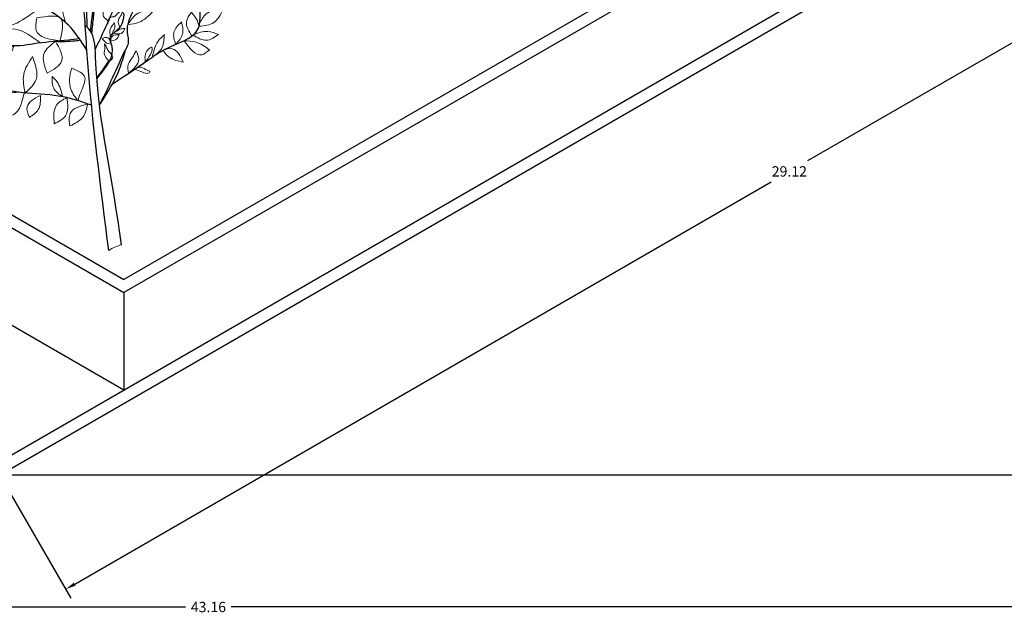
# Model space of a CAD drawing. Units: metres. Extents: x 12735 to 25554, y 20954 to 41989.
# Tile 10 of 15: x 12756 to 12773, y 20954 to 20964. Entities that reach past the tile are written whole.
import ezdxf

# ---------------------------------------------------------------- set-up
doc = ezdxf.new("R2010")
doc.units = ezdxf.units.M
doc.layers.get('Defpoints').update_dxf_attribs({"lineweight": 13})
for name, color, linetype, lineweight in [('A-ANNO-DIMS', 2, 'Continuous', 18), ('C-SITE', 8, 'Continuous', 25), ('TREES', 72, 'Continuous', 18)]:
    doc.layers.add(name, color=color, linetype=linetype, lineweight=lineweight)
doc.layers.add('STEM', color=32, linetype='Continuous')
doc.styles.get("Standard").update_dxf_attribs({"font": 'arial.ttf'})
doc.dimstyles.get("Standard").update_dxf_attribs({"dimtxt": 0.18, "dimasz": 0.18, "dimexe": 0.18, "dimexo": 0.0625, "dimgap": 0.09, "dimtad": 0, "dimtih": 1, "dimtoh": 1, "dimdec": 4, "dimzin": 0, "dimdsep": 46, "dimtxsty": 'Standard', "dimcen": 0.09, "dimadec": 0, "dimazin": 0, "dimtfac": 1, "dimtdec": 4, "dimtofl": 0, "dimtmove": 0, "dimatfit": 3, "dimfxl": 1, "dimtolj": 1, "dimtzin": 0, "dimarcsym": 0})

# ---------------------------------------------------------------- blocks, each defined once
blk = doc.blocks.new('TREES')
blk.add_line((12743.7, 20972.648), (12743.7, 20972.648))
at = {"layer": 'STEM'}
for points, knots in [([(12743.791, 20972.546), (12743.793, 20972.564), (12743.795, 20972.582), (12743.797, 20972.6), (12743.801, 20972.637), (12743.806, 20972.674), (12743.81, 20972.711), (12743.845, 20973.018), (12743.938, 20973.826), (12743.743, 20974.806), (12743.607, 20975.634), (12743.413, 20975.893), (12743.333, 20975.999)], [-0.164913, -0.164913, -0.164913, -0.164913, -0.110972, -0.110972, -0.110972, 0, 0, 0, 0.920963, 2.426088, 2.990404, 3.384799, 3.384799, 3.384799, 3.384799]), ([(12743.7, 20972.648), (12743.691, 20972.807), (12743.671, 20973.194), (12743.257, 20973.699), (12743.111, 20974.379), (12743.038, 20974.998), (12742.993, 20975.377), (12742.974, 20975.54)], [0, 0, 0, 0, 0.469346, 1.137622, 1.869488, 2.521439, 3.013071, 3.013071, 3.013071, 3.013071]), ([(12743.874, 20972.227), (12743.898, 20972.277), (12743.921, 20972.328), (12743.945, 20972.378), (12744.022, 20972.541), (12744.105, 20972.717), (12744.205, 20972.963), (12744.312, 20973.088), (12744.183, 20973.501), (12744.667, 20973.973), (12744.707, 20974.64), (12744.896, 20975.012), (12744.823, 20975.434), (12744.85, 20975.23), (12744.867, 20975.1)], [-0.166951, -0.166951, -0.166951, -0.166951, 0, 0, 0, 0.539768, 0.582066, 0.798222, 0.98781, 1.7696, 2.524754, 2.899414, 3.105113, 3.460848, 3.460848, 3.460848, 3.460848]), ([(12743.728, 20972.218), (12743.63, 20972.372), (12743.383, 20972.76), (12742.753, 20973.07), (12742.291, 20973.419), (12741.984, 20973.759), (12741.959, 20974.098), (12741.675, 20974.346), (12741.563, 20974.543), (12741.494, 20974.663)], [0, 0, 0, 0, 0.542161, 1.359078, 2.03444, 2.290187, 2.703676, 2.968549, 3.382864, 3.382864, 3.382864, 3.382864]), ([(12743.967, 20971.294), (12743.987, 20971.335), (12744.006, 20971.376), (12744.026, 20971.417), (12744.057, 20971.483), (12744.088, 20971.549), (12744.119, 20971.615), (12744.196, 20971.778), (12744.279, 20971.954), (12744.378, 20972.2), (12744.486, 20972.325), (12744.357, 20972.738), (12744.836, 20973.215), (12744.895, 20973.862), (12745.051, 20974.269), (12745.045, 20974.62), (12744.834, 20974.67), (12744.7, 20974.701)], [-0.355099, -0.355099, -0.355099, -0.355099, -0.218492, -0.218492, -0.218492, 0, 0, 0, 0.539768, 0.582066, 0.798222, 0.98781, 1.7696, 2.524754, 2.899414, 3.105113, 3.460848, 3.460848, 3.460848, 3.460848]), ([(12744.175, 20971.633), (12744.383, 20971.767), (12744.692, 20971.967), (12745.149, 20972.305), (12745.828, 20972.463), (12745.606, 20973.185), (12745.967, 20973.583), (12745.99, 20973.882), (12746.002, 20974.029)], [0, 0, 0, 0, 0.736164, 1.094646, 1.754618, 2.392389, 2.840214, 3.27091, 3.27091, 3.27091, 3.27091]), ([(12743.381, 20973.588), (12743.52, 20973.4), (12743.728, 20973.118), (12743.725, 20972.776), (12743.724, 20972.661), (12743.724, 20972.661), (12743.724, 20972.661), (12743.724, 20972.661), (12743.724, 20972.65), (12743.724, 20972.639), (12743.724, 20972.627)], [0, 0, 0, 0, 0.673099, 1.009429, 1.009429, 1.009429, 1.009429, 1.009429, 1.009429, 1.043412, 1.043412, 1.043412, 1.043412]), ([(12743.814, 20972.505), (12743.817, 20972.531), (12743.819, 20972.556), (12743.822, 20972.581), (12743.827, 20972.63), (12743.832, 20972.679), (12743.838, 20972.727), (12743.847, 20972.813), (12743.865, 20972.982), (12743.864, 20973.152), (12743.864, 20973.236)], [-0.2227932, -0.2227932, -0.2227932, -0.2227932, -0.1464713, -0.1464713, -0.1464713, 0, 0, 0, 0.2578951, 0.5103882, 0.5103882, 0.5103882, 0.5103882]), ([(12743.902, 20971.717), (12743.93, 20971.754), (12743.959, 20971.791), (12743.988, 20971.829), (12743.988, 20971.829), (12743.988, 20971.829), (12743.988, 20971.829), (12744.096, 20971.973), (12744.236, 20972.16), (12744.082, 20972.476), (12744.347, 20972.598), (12744.368, 20972.766), (12744.376, 20972.837)], [-0.129757, -0.129757, -0.129757, -0.129757, 0, 0, 0, 0, 0, 0, 0.485118, 0.62751, 0.913144, 1.120766, 1.120766, 1.120766, 1.120766]), ([(12744.111, 20968.725), (12743.967, 20969.837), (12743.799, 20971.142), (12743.712, 20972.453), (12743.7, 20972.648)], [0, 0, 0, 0, 3.359203, 3.944548, 3.944548, 3.944548, 3.944548]), ([(12744.332, 20968.825), (12744.189, 20969.936), (12743.871, 20971.161), (12743.872, 20972.51), (12743.7, 20972.648)], [0, 0, 0, 0, 3.359203, 3.972384, 3.972384, 3.972384, 3.972384]), ([(12743.597, 20972.418), (12743.533, 20972.41), (12743.292, 20972.379), (12742.889, 20972.351), (12742.364, 20972.241), (12741.803, 20972.489), (12741.157, 20972.302), (12740.698, 20972.258), (12740.474, 20972.237)], [0, 0, 0, 0, 0.193148, 0.727923, 1.218416, 1.762371, 2.471743, 3.152626, 3.152626, 3.152626, 3.152626]), ([(12743.181, 20972.372), (12743.296, 20972.37), (12743.441, 20972.368), (12743.583, 20972.39), (12743.613, 20972.395)], [0, 0, 0, 0, 0.3435042, 0.4329772, 0.4329772, 0.4329772, 0.4329772]), ([(12743.948, 20971.264), (12743.975, 20971.305), (12744.002, 20971.345), (12744.029, 20971.386), (12744.029, 20971.386), (12744.029, 20971.386), (12744.029, 20971.386), (12744.129, 20971.55), (12744.289, 20971.812), (12744.368, 20972.107), (12744.398, 20972.218)], [-0.148605, -0.148605, -0.148605, -0.148605, 0, 0, 0, 0, 0, 0, 0.572176, 0.914425, 0.914425, 0.914425, 0.914425]), ([(12743.901, 20971.729), (12743.929, 20971.768), (12743.958, 20971.808), (12743.986, 20971.847), (12743.986, 20971.847), (12743.986, 20971.847), (12743.986, 20971.847), (12744.02, 20971.892), (12744.062, 20971.951), (12744.099, 20972.014), (12744.107, 20972.028)], [-0.1467707, -0.1467707, -0.1467707, -0.1467707, 0, 0, 0, 0, 0, 0, 0.1684242, 0.2179474, 0.2179474, 0.2179474, 0.2179474]), ([(12743.81, 20971.258), (12743.646, 20971.316), (12743.283, 20971.443), (12742.486, 20971.453), (12741.888, 20971.61), (12741.494, 20971.714)], [0, 0, 0, 0, 0.519056, 1.146346, 2.366016, 2.366016, 2.366016, 2.366016])]:
    blk.add_open_spline(points, degree=3, knots=knots, dxfattribs=at)
blk.add_open_spline([(12744.644, 20971.941), (12744.672, 20971.961), (12744.701, 20971.98), (12744.73, 20972)], degree=3, dxfattribs=at)
at = {"layer": 'TREES'}
for points, knots in [([(12743.584, 20975.586), (12743.37, 20975.718), (12743.075, 20975.9), (12743.022, 20976.725), (12743.333, 20976.097), (12743.574, 20975.612)], [0, 0, 0, 0, 0.724771, 1.002271, 1.932196, 1.932196, 1.932196, 1.932196]), ([(12743.021, 20975.14), (12742.985, 20975.224), (12742.928, 20975.356), (12742.766, 20975.539), (12742.854, 20975.638), (12742.901, 20975.69)], [0, 0, 0, 0, 0.2845416, 0.4465287, 0.6279758, 0.6279758, 0.6279758, 0.6279758]), ([(12743.021, 20975.14), (12743.019, 20975.277), (12743.016, 20975.483), (12742.921, 20975.662), (12742.889, 20975.721)], [0, 0, 0, 0, 0.4023849, 0.6031293, 0.6031293, 0.6031293, 0.6031293]), ([(12743.718, 20974.979), (12743.671, 20975.164), (12743.598, 20975.454), (12743.323, 20975.534), (12743.223, 20975.563)], [0, 0, 0, 0, 0.519429, 0.8155501, 0.8155501, 0.8155501, 0.8155501]), ([(12743.223, 20975.563), (12743.266, 20975.448), (12743.36, 20975.195), (12743.592, 20975.055), (12743.718, 20974.979)], [0, 0, 0, 0, 0.3595778, 0.7860105, 0.7860105, 0.7860105, 0.7860105]), ([(12743.737, 20974.871), (12743.729, 20975.055), (12743.718, 20975.333), (12743.914, 20975.516), (12743.981, 20975.578)], [0, 0, 0, 0, 0.5134638, 0.7779111, 0.7779111, 0.7779111, 0.7779111]), ([(12743.737, 20974.871), (12743.801, 20974.971), (12743.939, 20975.186), (12743.966, 20975.441), (12743.981, 20975.578)], [0, 0, 0, 0, 0.351068, 0.7565079, 0.7565079, 0.7565079, 0.7565079]), ([(12744.796, 20974.806), (12744.757, 20974.909), (12744.688, 20975.088), (12744.514, 20975.28), (12744.523, 20975.414), (12744.526, 20975.464)], [0, 0, 0, 0, 0.3323117, 0.5782809, 0.7232611, 0.7232611, 0.7232611, 0.7232611]), ([(12744.805, 20974.813), (12744.804, 20974.918), (12744.803, 20975.076), (12744.822, 20975.37), (12744.643, 20975.427), (12744.526, 20975.464)], [0, 0, 0, 0, 0.3224266, 0.4885617, 0.8037384, 0.8037384, 0.8037384, 0.8037384]), ([(12741.648, 20974.411), (12741.519, 20974.547), (12741.281, 20974.798), (12741.642, 20974.995), (12741.673, 20975.511), (12741.684, 20975.149), (12741.787, 20975.033), (12741.768, 20974.824), (12741.781, 20974.575), (12741.641, 20974.411), (12741.569, 20974.326)], [0, 0, 0, 0, 0.446457, 0.821839, 1.096823, 1.294203, 1.491123, 1.594729, 1.894892, 2.216107, 2.216107, 2.216107, 2.216107]), ([(12743.07, 20974.733), (12742.98, 20974.863), (12742.848, 20975.053), (12742.433, 20975.446), (12742.649, 20974.915), (12742.651, 20974.573), (12742.961, 20974.576), (12743.034, 20974.678), (12743.071, 20974.73)], [0, 0, 0, 0, 0.54832, 0.799685, 1.166614, 1.565159, 1.742127, 1.925713, 1.925713, 1.925713, 1.925713]), ([(12743.031, 20975.058), (12743.048, 20975.139), (12743.077, 20975.281), (12743.184, 20975.377), (12743.231, 20975.418)], [0, 0, 0, 0, 0.2398723, 0.4207027, 0.4207027, 0.4207027, 0.4207027]), ([(12743.037, 20975.007), (12743.075, 20975.058), (12743.166, 20975.181), (12743.207, 20975.33), (12743.231, 20975.418)], [0, 0, 0, 0, 0.1895117, 0.457602, 0.457602, 0.457602, 0.457602]), ([(12744.796, 20974.806), (12744.882, 20974.878), (12745.017, 20974.992), (12745.211, 20975.15), (12745.228, 20975.277), (12745.236, 20975.337)], [0, 0, 0, 0, 0.3416822, 0.5370609, 0.7122352, 0.7122352, 0.7122352, 0.7122352]), ([(12744.839, 20974.951), (12744.859, 20975.055), (12744.903, 20975.272), (12745.122, 20975.315), (12745.236, 20975.337)], [0, 0, 0, 0, 0.2913456, 0.6064398, 0.6064398, 0.6064398, 0.6064398]), ([(12743.814, 20974.4), (12743.798, 20974.494), (12743.764, 20974.693), (12744.115, 20975.006), (12744.156, 20974.79), (12744.01, 20974.677), (12743.989, 20974.434), (12743.864, 20974.438), (12743.809, 20974.439)], [0, 0, 0, 0, 0.311146, 0.650746, 0.669061, 0.940573, 1.125337, 1.270427, 1.270427, 1.270427, 1.270427]), ([(12743.191, 20974.047), (12743.14, 20974.139), (12743.026, 20974.346), (12743.367, 20974.877), (12743.354, 20974.597), (12743.309, 20974.413), (12743.358, 20974.125), (12743.218, 20974.059), (12743.191, 20974.047)], [0, 0, 0, 0, 0.337622, 0.758697, 0.837919, 1.040495, 1.406258, 1.489574, 1.489574, 1.489574, 1.489574]), ([(12744.509, 20973.941), (12744.486, 20974.093), (12744.451, 20974.322), (12744.425, 20974.623), (12744.504, 20974.731), (12744.534, 20974.773)], [0, 0, 0, 0, 0.4681587, 0.7056034, 0.8580265, 0.8580265, 0.8580265, 0.8580265]), ([(12744.534, 20974.773), (12744.556, 20974.698), (12744.634, 20974.425), (12744.562, 20974.144), (12744.509, 20973.941)], [0, 0, 0, 0, 0.2327329, 0.8431329, 0.8431329, 0.8431329, 0.8431329]), ([(12742.028, 20973.754), (12742.003, 20973.912), (12741.953, 20974.218), (12742.174, 20974.414), (12742.283, 20974.81), (12742.258, 20974.48), (12742.304, 20974.323), (12742.246, 20974.069), (12742.227, 20973.932), (12742.006, 20973.671), (12742.066, 20973.72), (12742.075, 20973.727)], [0, 0, 0, 0, 0.436736, 0.842969, 1.012738, 1.21393, 1.403734, 1.613178, 1.897283, 2.067562, 2.097274, 2.097274, 2.097274, 2.097274]), ([(12743.835, 20974.249), (12743.789, 20974.346), (12743.724, 20974.484), (12743.556, 20974.594), (12743.468, 20974.601), (12743.424, 20974.604)], [0, 0, 0, 0, 0.3158223, 0.4463774, 0.5774617, 0.5774617, 0.5774617, 0.5774617]), ([(12743.424, 20974.604), (12743.442, 20974.527), (12743.487, 20974.324), (12743.715, 20974.191), (12743.841, 20974.206), (12743.841, 20974.206)], [0, 0, 0, 0, 0.2361186, 0.6165307, 0.6167763, 0.6167763, 0.6167763, 0.6167763]), ([(12744.554, 20973.975), (12744.669, 20974.016), (12744.893, 20974.094), (12745.019, 20974.421), (12745.06, 20974.624), (12745.08, 20974.72)], [0, 0, 0, 0, 0.348929, 0.678298, 0.9763146, 0.9763146, 0.9763146, 0.9763146]), ([(12744.618, 20974.118), (12744.717, 20974.268), (12744.844, 20974.462), (12745.022, 20974.606), (12745.062, 20974.638)], [0, 0, 0, 0, 0.5333846, 0.686651, 0.686651, 0.686651, 0.686651]), ([(12744.97, 20974.043), (12744.931, 20974.146), (12744.862, 20974.325), (12744.688, 20974.517), (12744.697, 20974.651), (12744.7, 20974.701)], [0, 0, 0, 0, 0.3323117, 0.5782809, 0.7232611, 0.7232611, 0.7232611, 0.7232611]), ([(12745.957, 20973.706), (12745.908, 20973.835), (12745.798, 20974.123), (12745.864, 20974.427), (12745.9, 20974.594)], [0, 0, 0, 0, 0.4051126, 0.906838, 0.906838, 0.906838, 0.906838]), ([(12745.9, 20974.594), (12745.955, 20974.471), (12746.037, 20974.287), (12746.01, 20974.092), (12746.002, 20974.029)], [0, 0, 0, 0, 0.3943838, 0.5836156, 0.5836156, 0.5836156, 0.5836156]), ([(12744.97, 20974.043), (12745.056, 20974.115), (12745.191, 20974.229), (12745.385, 20974.387), (12745.402, 20974.514), (12745.41, 20974.574)], [0, 0, 0, 0, 0.3416822, 0.5370609, 0.7122352, 0.7122352, 0.7122352, 0.7122352]), ([(12745.013, 20974.188), (12745.033, 20974.292), (12745.077, 20974.509), (12745.296, 20974.552), (12745.41, 20974.574)], [0, 0, 0, 0, 0.2913456, 0.6064398, 0.6064398, 0.6064398, 0.6064398]), ([(12741.943, 20974.016), (12741.835, 20974.13), (12741.594, 20974.382), (12741.272, 20973.991), (12740.687, 20974.27), (12741.289, 20973.836), (12741.63, 20973.742), (12741.878, 20973.799), (12742.016, 20973.831)], [0, 0, 0, 0, 0.397812, 0.88569, 1.156328, 1.66735, 1.991498, 2.394837, 2.394837, 2.394837, 2.394837]), ([(12743.128, 20974.182), (12743.019, 20974.275), (12742.841, 20974.427), (12742.65, 20974.313), (12742.577, 20974.27)], [0, 0, 0, 0, 0.3785086, 0.6144536, 0.6144536, 0.6144536, 0.6144536]), ([(12742.577, 20974.27), (12742.635, 20974.174), (12742.755, 20973.977), (12743.187, 20974.003), (12743.173, 20974.131), (12743.172, 20974.137)], [0, 0, 0, 0, 0.3386751, 0.6999446, 0.7185805, 0.7185805, 0.7185805, 0.7185805]), ([(12745.785, 20973.361), (12745.68, 20973.449), (12745.404, 20973.684), (12745.451, 20974.057), (12745.481, 20974.288)], [0, 0, 0, 0, 0.391493, 1.034106, 1.034106, 1.034106, 1.034106]), ([(12745.481, 20974.288), (12745.577, 20974.138), (12745.76, 20973.855), (12745.777, 20973.519), (12745.785, 20973.361)], [0, 0, 0, 0, 0.5245256, 0.9915723, 0.9915723, 0.9915723, 0.9915723]), ([(12743.879, 20973.555), (12743.816, 20973.752), (12743.731, 20974.021), (12743.982, 20974.067), (12744.068, 20974.224), (12744.006, 20973.984), (12744.093, 20973.824), (12743.961, 20973.709), (12743.879, 20973.638)], [0, 0, 0, 0, 0.469961, 0.638827, 0.705595, 0.853148, 1.022788, 1.296962, 1.296962, 1.296962, 1.296962]), ([(12744.356, 20973.647), (12744.309, 20973.708), (12744.202, 20973.846), (12744.245, 20974.018), (12744.268, 20974.113)], [0, 0, 0, 0, 0.2209277, 0.4981889, 0.4981889, 0.4981889, 0.4981889]), ([(12744.268, 20974.113), (12744.323, 20974.065), (12744.46, 20973.94), (12744.395, 20973.758), (12744.356, 20973.647)], [0, 0, 0, 0, 0.203616, 0.5174389, 0.5174389, 0.5174389, 0.5174389]), ([(12742.389, 20973.356), (12742.341, 20973.437), (12742.234, 20973.617), (12742.458, 20973.799), (12742.48, 20973.946), (12742.486, 20973.991)], [0, 0, 0, 0, 0.251735, 0.5591808, 0.6938707, 0.6938707, 0.6938707, 0.6938707]), ([(12742.486, 20973.991), (12742.542, 20973.959), (12742.68, 20973.88), (12742.598, 20973.572), (12742.464, 20973.433), (12742.389, 20973.356)], [0, 0, 0, 0, 0.1746142, 0.4385715, 0.7703441, 0.7703441, 0.7703441, 0.7703441]), ([(12743.381, 20973.588), (12743.369, 20973.67), (12743.344, 20973.833), (12743.453, 20973.958), (12743.508, 20974.02)], [0, 0, 0, 0, 0.2360196, 0.4713289, 0.4713289, 0.4713289, 0.4713289]), ([(12743.381, 20973.588), (12743.434, 20973.649), (12743.541, 20973.774), (12743.519, 20973.937), (12743.508, 20974.02)], [0, 0, 0, 0, 0.2309694, 0.4699481, 0.4699481, 0.4699481, 0.4699481]), ([(12744.683, 20973.178), (12744.66, 20973.33), (12744.625, 20973.559), (12744.599, 20973.86), (12744.677, 20973.968), (12744.708, 20974.01)], [0, 0, 0, 0, 0.4681587, 0.7056034, 0.8580265, 0.8580265, 0.8580265, 0.8580265]), ([(12744.708, 20974.01), (12744.73, 20973.935), (12744.807, 20973.662), (12744.735, 20973.381), (12744.683, 20973.178)], [0, 0, 0, 0, 0.2327329, 0.8431329, 0.8431329, 0.8431329, 0.8431329]), ([(12744.728, 20973.213), (12744.843, 20973.253), (12745.067, 20973.331), (12745.193, 20973.658), (12745.234, 20973.861), (12745.254, 20973.957)], [0, 0, 0, 0, 0.348929, 0.678298, 0.9763146, 0.9763146, 0.9763146, 0.9763146]), ([(12743.364, 20973.617), (12743.288, 20973.661), (12743.124, 20973.754), (12742.939, 20973.715), (12742.84, 20973.694)], [0, 0, 0, 0, 0.2535199, 0.5460217, 0.5460217, 0.5460217, 0.5460217]), ([(12743.851, 20973.09), (12743.747, 20973.196), (12743.578, 20973.368), (12743.647, 20973.644), (12743.671, 20973.769), (12743.679, 20973.81)], [0, 0, 0, 0, 0.4076044, 0.6640272, 0.7921335, 0.7921335, 0.7921335, 0.7921335]), ([(12743.679, 20973.81), (12743.708, 20973.778), (12743.776, 20973.703), (12743.798, 20973.443), (12743.829, 20973.238), (12743.851, 20973.09)], [0, 0, 0, 0, 0.125659, 0.2981213, 0.7527794, 0.7527794, 0.7527794, 0.7527794]), ([(12744.792, 20973.355), (12744.891, 20973.505), (12745.018, 20973.699), (12745.196, 20973.843), (12745.236, 20973.876)], [0, 0, 0, 0, 0.5333846, 0.686651, 0.686651, 0.686651, 0.686651]), ([(12742.221, 20973.506), (12741.989, 20973.602), (12741.674, 20973.731), (12741.536, 20973.471), (12741.5, 20973.404)], [0, 0, 0, 0, 0.6060397, 0.8197481, 0.8197481, 0.8197481, 0.8197481]), ([(12743.253, 20972.784), (12743.147, 20972.854), (12742.919, 20973.005), (12742.8, 20973.728), (12742.973, 20973.491), (12743.022, 20973.422)], [0, 0, 0, 0, 0.420416, 0.90702, 1.103207, 1.103207, 1.103207, 1.103207]), ([(12742.84, 20973.694), (12742.956, 20973.634), (12743.128, 20973.545), (12743.306, 20973.6), (12743.364, 20973.617)], [0, 0, 0, 0, 0.369417, 0.546183, 0.546183, 0.546183, 0.546183]), ([(12744.268, 20973.425), (12744.32, 20973.505), (12744.424, 20973.666), (12744.615, 20973.662), (12744.711, 20973.66)], [0, 0, 0, 0, 0.2669279, 0.5349854, 0.5349854, 0.5349854, 0.5349854]), ([(12744.268, 20973.425), (12744.336, 20973.433), (12744.51, 20973.454), (12744.635, 20973.582), (12744.711, 20973.66)], [0, 0, 0, 0, 0.1990667, 0.5143408, 0.5143408, 0.5143408, 0.5143408]), ([(12741.493, 20973.429), (12741.634, 20973.396), (12741.906, 20973.333), (12742.16, 20973.449), (12742.283, 20973.505)], [0, 0, 0, 0, 0.420024, 0.8136231, 0.8136231, 0.8136231, 0.8136231]), ([(12743.022, 20973.422), (12743.059, 20973.426), (12743.334, 20973.456), (12743.256, 20972.956), (12743.349, 20972.723), (12743.36, 20972.696)], [0, 0, 0, 0, 0.1039343, 0.7792863, 0.8705393, 0.8705393, 0.8705393, 0.8705393]), ([(12743.864, 20973.236), (12743.891, 20973.272), (12743.952, 20973.35), (12744.077, 20973.438), (12744.058, 20973.527), (12744.051, 20973.558)], [0, 0, 0, 0, 0.1377377, 0.3031534, 0.3935537, 0.3935537, 0.3935537, 0.3935537]), ([(12743.866, 20973.267), (12743.872, 20973.352), (12743.881, 20973.49), (12744.004, 20973.539), (12744.051, 20973.558)], [0, 0, 0, 0, 0.2295676, 0.3730638, 0.3730638, 0.3730638, 0.3730638]), ([(12745.697, 20972.996), (12745.547, 20972.999), (12745.238, 20973.004), (12745.268, 20973.314), (12745.283, 20973.473)], [0, 0, 0, 0, 0.3799868, 0.779071, 0.779071, 0.779071, 0.779071]), ([(12745.283, 20973.473), (12745.354, 20973.458), (12745.585, 20973.409), (12745.651, 20973.165), (12745.697, 20972.996)], [0, 0, 0, 0, 0.2074949, 0.6743984, 0.6743984, 0.6743984, 0.6743984]), ([(12741.595, 20972.406), (12741.523, 20972.496), (12741.318, 20972.752), (12741.336, 20973.087), (12741.348, 20973.304)], [0, 0, 0, 0, 0.3390919, 0.9589007, 0.9589007, 0.9589007, 0.9589007]), ([(12741.348, 20973.304), (12741.406, 20973.227), (12741.6, 20972.969), (12741.591, 20972.637), (12741.585, 20972.405)], [0, 0, 0, 0, 0.2865181, 0.9509807, 0.9509807, 0.9509807, 0.9509807]), ([(12743.621, 20973.151), (12743.561, 20973.233), (12743.473, 20973.354), (12743.333, 20973.334), (12743.288, 20973.327)], [0, 0, 0, 0, 0.2726158, 0.4022356, 0.4022356, 0.4022356, 0.4022356]), ([(12743.288, 20973.327), (12743.325, 20973.265), (12743.399, 20973.138), (12743.546, 20973.147), (12743.621, 20973.151)], [0, 0, 0, 0, 0.199886, 0.4070645, 0.4070645, 0.4070645, 0.4070645]), ([(12744.53, 20972.884), (12744.482, 20972.945), (12744.376, 20973.084), (12744.419, 20973.255), (12744.442, 20973.351)], [0, 0, 0, 0, 0.2209277, 0.4981889, 0.4981889, 0.4981889, 0.4981889]), ([(12744.442, 20973.351), (12744.496, 20973.302), (12744.634, 20973.177), (12744.569, 20972.995), (12744.53, 20972.884)], [0, 0, 0, 0, 0.203616, 0.5174389, 0.5174389, 0.5174389, 0.5174389]), ([(12745.697, 20972.996), (12745.724, 20973.08), (12745.77, 20973.226), (12745.915, 20973.262), (12745.976, 20973.277)], [0, 0, 0, 0, 0.2439478, 0.4222058, 0.4222058, 0.4222058, 0.4222058]), ([(12745.697, 20972.996), (12745.764, 20973.024), (12745.897, 20973.078), (12745.95, 20973.211), (12745.976, 20973.277)], [0, 0, 0, 0, 0.2073861, 0.4117039, 0.4117039, 0.4117039, 0.4117039]), ([(12742.983, 20972.961), (12742.799, 20973.009), (12742.463, 20973.098), (12742.071, 20972.928), (12741.893, 20972.798), (12741.839, 20972.759)], [0, 0, 0, 0, 0.553894, 1.01265, 1.215779, 1.215779, 1.215779, 1.215779]), ([(12743.669, 20972.977), (12743.606, 20973.025), (12743.504, 20973.102), (12743.398, 20973.043), (12743.358, 20973.021)], [0, 0, 0, 0, 0.2119595, 0.340544, 0.340544, 0.340544, 0.340544]), ([(12744.074, 20972.655), (12744.086, 20972.673), (12744.124, 20972.731), (12743.998, 20972.782), (12744.014, 20972.867), (12744.011, 20972.925), (12744.052, 20972.944), (12744.07, 20973.015), (12743.988, 20973.027), (12743.97, 20973.091), (12744.03, 20973.11), (12744.072, 20973.132), (12744.097, 20973.169), (12744.133, 20973.163), (12744.172, 20973.164), (12744.216, 20973.136), (12744.296, 20973.17), (12744.282, 20973.105), (12744.259, 20973.057), (12744.341, 20973.048), (12744.328, 20972.986), (12744.32, 20972.935), (12744.299, 20972.884), (12744.258, 20972.852), (12744.236, 20972.821), (12744.215, 20972.805), (12744.179, 20972.793), (12744.139, 20972.807), (12744.095, 20972.746), (12744.111, 20972.739), (12744.111, 20972.739)], [0, 0, 0, 0, 0.055886, 0.185472, 0.25227, 0.305988, 0.338368, 0.378405, 0.48523, 0.4997, 0.565031, 0.618654, 0.656012, 0.680602, 0.71942, 0.77395, 0.836088, 0.890088, 0.913694, 0.979696, 1.032481, 1.0683, 1.142133, 1.186825, 1.224162, 1.25438, 1.26551, 1.333296, 1.383591, 1.385324, 1.385324, 1.385324, 1.385324]), ([(12741.839, 20972.759), (12741.949, 20972.7), (12742.323, 20972.501), (12742.684, 20972.786), (12742.939, 20972.987)], [0, 0, 0, 0, 0.355589, 1.206871, 1.206871, 1.206871, 1.206871]), ([(12743.358, 20973.021), (12743.426, 20972.983), (12743.527, 20972.926), (12743.633, 20972.964), (12743.669, 20972.977)], [0, 0, 0, 0, 0.2166399, 0.3265492, 0.3265492, 0.3265492, 0.3265492]), ([(12744.299, 20972.615), (12744.284, 20972.657), (12744.255, 20972.734), (12744.322, 20972.816), (12744.34, 20972.869), (12744.347, 20972.89)], [0, 0, 0, 0, 0.1248577, 0.2264879, 0.2926557, 0.2926557, 0.2926557, 0.2926557]), ([(12744.442, 20972.662), (12744.494, 20972.743), (12744.598, 20972.903), (12744.789, 20972.899), (12744.885, 20972.897)], [0, 0, 0, 0, 0.2669279, 0.5349854, 0.5349854, 0.5349854, 0.5349854]), ([(12744.442, 20972.662), (12744.51, 20972.671), (12744.684, 20972.691), (12744.809, 20972.819), (12744.885, 20972.897)], [0, 0, 0, 0, 0.1990667, 0.5143408, 0.5143408, 0.5143408, 0.5143408]), ([(12745.557, 20972.46), (12745.505, 20972.545), (12745.415, 20972.69), (12745.509, 20972.826), (12745.548, 20972.882)], [0, 0, 0, 0, 0.2672291, 0.4594629, 0.4594629, 0.4594629, 0.4594629]), ([(12745.548, 20972.882), (12745.623, 20972.785), (12745.735, 20972.639), (12745.619, 20972.519), (12745.581, 20972.479)], [0, 0, 0, 0, 0.3063433, 0.4579535, 0.4579535, 0.4579535, 0.4579535]), ([(12745.681, 20972.634), (12745.776, 20972.643), (12745.97, 20972.661), (12746.056, 20972.838), (12746.1, 20972.929)], [0, 0, 0, 0, 0.2646598, 0.5464061, 0.5464061, 0.5464061, 0.5464061]), ([(12745.691, 20972.679), (12745.723, 20972.743), (12745.803, 20972.904), (12745.989, 20972.919), (12746.1, 20972.929)], [0, 0, 0, 0, 0.2025395, 0.5100625, 0.5100625, 0.5100625, 0.5100625]), ([(12741.358, 20972.366), (12741.291, 20972.434), (12741.162, 20972.564), (12740.909, 20972.646), (12740.492, 20972.989), (12740.719, 20972.381), (12740.905, 20972.253), (12741.437, 20972.382), (12741.361, 20972.366), (12741.358, 20972.366)], [0, 0, 0, 0, 0.274554, 0.529523, 0.902439, 1.220606, 1.740632, 1.953969, 1.962894, 1.962894, 1.962894, 1.962894]), ([(12743.257, 20972.379), (12743.071, 20972.409), (12742.794, 20972.453), (12742.842, 20972.698), (12742.858, 20972.779)], [0, 0, 0, 0, 0.4478858, 0.6692237, 0.6692237, 0.6692237, 0.6692237]), ([(12742.858, 20972.779), (12743.034, 20972.81), (12743.375, 20972.87), (12743.295, 20972.539), (12743.257, 20972.379)], [0, 0, 0, 0, 0.4156133, 0.8046117, 0.8046117, 0.8046117, 0.8046117]), ([(12745.276, 20972.317), (12745.252, 20972.391), (12745.204, 20972.544), (12745.32, 20972.655), (12745.379, 20972.712)], [0, 0, 0, 0, 0.2148949, 0.4418034, 0.4418034, 0.4418034, 0.4418034]), ([(12745.276, 20972.317), (12745.329, 20972.378), (12745.429, 20972.493), (12745.395, 20972.642), (12745.379, 20972.712)], [0, 0, 0, 0, 0.2259484, 0.4304915, 0.4304915, 0.4304915, 0.4304915]), ([(12740.645, 20972.254), (12740.532, 20972.287), (12740.33, 20972.345), (12740.37, 20972.543), (12740.387, 20972.63)], [0, 0, 0, 0, 0.300298, 0.5327787, 0.5327787, 0.5327787, 0.5327787]), ([(12740.387, 20972.63), (12740.446, 20972.602), (12740.598, 20972.53), (12740.627, 20972.359), (12740.645, 20972.254)], [0, 0, 0, 0, 0.1847401, 0.4807235, 0.4807235, 0.4807235, 0.4807235]), ([(12742.916, 20972.343), (12742.772, 20972.452), (12742.448, 20972.697), (12742.076, 20972.511), (12741.869, 20972.407)], [0, 0, 0, 0, 0.501704, 1.133573, 1.133573, 1.133573, 1.133573]), ([(12744.14, 20972.455), (12744.129, 20972.498), (12744.112, 20972.571), (12744.173, 20972.643), (12744.195, 20972.684), (12744.204, 20972.7)], [0, 0, 0, 0, 0.124617, 0.2107396, 0.2658134, 0.2658134, 0.2658134, 0.2658134]), ([(12744.14, 20972.455), (12744.155, 20972.485), (12744.181, 20972.535), (12744.225, 20972.615), (12744.212, 20972.669), (12744.204, 20972.7)], [0, 0, 0, 0, 0.1037237, 0.1704768, 0.2630686, 0.2630686, 0.2630686, 0.2630686]), ([(12744.192, 20972.515), (12744.244, 20972.502), (12744.335, 20972.479), (12744.372, 20972.56), (12744.387, 20972.593)], [0, 0, 0, 0, 0.1401829, 0.239855, 0.239855, 0.239855, 0.239855]), ([(12744.25, 20972.55), (12744.272, 20972.566), (12744.314, 20972.595), (12744.364, 20972.594), (12744.387, 20972.593)], [0, 0, 0, 0, 0.0790636, 0.1468534, 0.1468534, 0.1468534, 0.1468534]), ([(12745.582, 20972.481), (12745.667, 20972.516), (12745.814, 20972.576), (12745.958, 20972.516), (12746.019, 20972.491)], [0, 0, 0, 0, 0.2625898, 0.453199, 0.453199, 0.453199, 0.453199]), ([(12741.223, 20971.823), (12741.319, 20971.881), (12741.571, 20972.033), (12741.755, 20972.264), (12741.869, 20972.407)], [0, 0, 0, 0, 0.3340001, 0.876507, 0.876507, 0.876507, 0.876507]), ([(12741.595, 20972.406), (12741.515, 20972.319), (12741.356, 20972.147), (12741.267, 20971.93), (12741.223, 20971.823)], [0, 0, 0, 0, 0.3521388, 0.6963584, 0.6963584, 0.6963584, 0.6963584]), ([(12743.181, 20972.372), (12743.094, 20972.305), (12742.907, 20972.162), (12742.991, 20971.938), (12743.035, 20971.819)], [0, 0, 0, 0, 0.2977969, 0.6372286, 0.6372286, 0.6372286, 0.6372286]), ([(12743.035, 20971.819), (12743.147, 20971.88), (12743.383, 20972.009), (12743.25, 20972.247), (12743.181, 20972.372)], [0, 0, 0, 0, 0.3275492, 0.688496, 0.688496, 0.688496, 0.688496]), ([(12744.145, 20972.348), (12744.132, 20972.384), (12744.105, 20972.455), (12744.032, 20972.434), (12743.996, 20972.423)], [0, 0, 0, 0, 0.098996, 0.196743, 0.196743, 0.196743, 0.196743]), ([(12743.996, 20972.423), (12744.027, 20972.377), (12744.069, 20972.315), (12744.13, 20972.341), (12744.146, 20972.347)], [0, 0, 0, 0, 0.1368513, 0.185287, 0.185287, 0.185287, 0.185287]), ([(12744.137, 20972.378), (12744.147, 20972.414), (12744.168, 20972.49), (12744.249, 20972.485), (12744.292, 20972.483)], [0, 0, 0, 0, 0.0982704, 0.2114853, 0.2114853, 0.2114853, 0.2114853]), ([(12744.137, 20972.378), (12744.171, 20972.382), (12744.241, 20972.388), (12744.274, 20972.45), (12744.292, 20972.483)], [0, 0, 0, 0, 0.0955829, 0.1975677, 0.1975677, 0.1975677, 0.1975677]), ([(12744.868, 20972.097), (12744.937, 20972.148), (12745.072, 20972.246), (12745.072, 20972.413), (12745.073, 20972.494)], [0, 0, 0, 0, 0.2403434, 0.4714363, 0.4714363, 0.4714363, 0.4714363]), ([(12744.868, 20972.097), (12744.895, 20972.212), (12744.931, 20972.363), (12745.046, 20972.458), (12745.074, 20972.481)], [0, 0, 0, 0, 0.3374321, 0.4432568, 0.4432568, 0.4432568, 0.4432568]), ([(12745.422, 20972.381), (12745.493, 20972.379), (12745.657, 20972.373), (12745.791, 20972.276), (12745.866, 20972.222)], [0, 0, 0, 0, 0.2087211, 0.4811791, 0.4811791, 0.4811791, 0.4811791]), ([(12745.422, 20972.381), (12745.521, 20972.247), (12745.661, 20972.058), (12745.82, 20972.185), (12745.866, 20972.222)], [0, 0, 0, 0, 0.3912381, 0.5526272, 0.5526272, 0.5526272, 0.5526272]), ([(12745.582, 20972.481), (12745.658, 20972.433), (12745.808, 20972.341), (12745.95, 20972.442), (12746.019, 20972.491)], [0, 0, 0, 0, 0.2451587, 0.4783488, 0.4783488, 0.4783488, 0.4783488]), ([(12740.645, 20972.254), (12740.54, 20972.264), (12740.318, 20972.286), (12740.252, 20972.07), (12740.216, 20971.955)], [0, 0, 0, 0, 0.2808571, 0.5946199, 0.5946199, 0.5946199, 0.5946199]), ([(12740.216, 20971.955), (12740.344, 20971.984), (12740.536, 20972.026), (12740.618, 20972.197), (12740.645, 20972.254)], [0, 0, 0, 0, 0.3624795, 0.5464116, 0.5464116, 0.5464116, 0.5464116]), ([(12740.757, 20972.265), (12740.712, 20972.237), (12740.573, 20972.15), (12740.673, 20971.993), (12740.741, 20971.887)], [0, 0, 0, 0, 0.1417373, 0.4445248, 0.4445248, 0.4445248, 0.4445248]), ([(12740.741, 20971.887), (12740.783, 20971.937), (12740.878, 20972.054), (12740.801, 20972.189), (12740.757, 20972.265)], [0, 0, 0, 0, 0.1798963, 0.4162104, 0.4162104, 0.4162104, 0.4162104]), ([(12742.453, 20972.29), (12742.257, 20972.189), (12741.999, 20972.056), (12742.001, 20971.792), (12742.002, 20971.729)], [0, 0, 0, 0, 0.5792647, 0.7616052, 0.7616052, 0.7616052, 0.7616052]), ([(12742.002, 20971.729), (12742.108, 20971.788), (12742.333, 20971.914), (12742.411, 20972.161), (12742.453, 20972.29)], [0, 0, 0, 0, 0.3533474, 0.7448355, 0.7448355, 0.7448355, 0.7448355]), ([(12744.116, 20972.018), (12744.075, 20972.065), (12744.007, 20972.143), (12744.05, 20972.231), (12744.028, 20972.351), (12744.072, 20972.271), (12744.09, 20972.201), (12744.221, 20972.106), (12744.146, 20972.042), (12744.116, 20972.018)], [0, 0, 0, 0, 0.1633748, 0.2727914, 0.3326965, 0.376171, 0.4524353, 0.6040881, 0.701786, 0.701786, 0.701786, 0.701786]), ([(12744.455, 20971.815), (12744.445, 20971.868), (12744.427, 20971.97), (12744.523, 20972.088), (12744.564, 20972.169), (12744.585, 20972.208)], [0, 0, 0, 0, 0.1538132, 0.2966411, 0.4292928, 0.4292928, 0.4292928, 0.4292928]), ([(12744.455, 20971.815), (12744.544, 20971.891), (12744.679, 20972.008), (12744.609, 20972.157), (12744.585, 20972.208)], [0, 0, 0, 0, 0.3019229, 0.4589929, 0.4589929, 0.4589929, 0.4589929]), ([(12744.746, 20972.012), (12744.742, 20972.047), (12744.733, 20972.118), (12744.771, 20972.218), (12744.826, 20972.252), (12744.849, 20972.268)], [0, 0, 0, 0, 0.1066556, 0.2131282, 0.2966333, 0.2966333, 0.2966333, 0.2966333]), ([(12744.746, 20972.012), (12744.773, 20972.045), (12744.822, 20972.105), (12744.891, 20972.268), (12744.848, 20972.268), (12744.847, 20972.268)], [0, 0, 0, 0, 0.1585708, 0.2833525, 0.285588, 0.285588, 0.285588, 0.285588]), ([(12745.053, 20972.215), (12745.111, 20972.233), (12745.273, 20972.284), (12745.353, 20972.117), (12745.405, 20972.009)], [0, 0, 0, 0, 0.1646898, 0.4645687, 0.4645687, 0.4645687, 0.4645687]), ([(12745.053, 20972.215), (12745.087, 20972.171), (12745.174, 20972.057), (12745.317, 20972.027), (12745.405, 20972.009)], [0, 0, 0, 0, 0.1638697, 0.4194041, 0.4194041, 0.4194041, 0.4194041]), ([(12742.652, 20971.471), (12742.63, 20971.58), (12742.585, 20971.809), (12742.714, 20972.005), (12742.781, 20972.107)], [0, 0, 0, 0, 0.3207709, 0.6721329, 0.6721329, 0.6721329, 0.6721329]), ([(12742.652, 20971.471), (12742.732, 20971.545), (12742.92, 20971.718), (12742.832, 20971.965), (12742.781, 20972.107)], [0, 0, 0, 0, 0.3028446, 0.7080533, 0.7080533, 0.7080533, 0.7080533]), ([(12742.314, 20971.521), (12742.225, 20971.627), (12742.039, 20971.851), (12741.746, 20971.851), (12741.593, 20971.851)], [0, 0, 0, 0, 0.3968877, 0.8302181, 0.8302181, 0.8302181, 0.8302181]), ([(12741.593, 20971.851), (12741.666, 20971.793), (12741.821, 20971.668), (12742.447, 20971.471), (12742.312, 20971.521), (12742.311, 20971.521)], [0, 0, 0, 0, 0.3696351, 0.7965164, 0.7990281, 0.7990281, 0.7990281, 0.7990281]), ([(12743.566, 20971.341), (12743.514, 20971.414), (12743.424, 20971.54), (12743.418, 20971.749), (12743.449, 20971.857), (12743.463, 20971.904)], [0, 0, 0, 0, 0.2632417, 0.4527737, 0.6011812, 0.6011812, 0.6011812, 0.6011812]), ([(12743.463, 20971.904), (12743.567, 20971.861), (12743.772, 20971.775), (12743.623, 20971.516), (12743.587, 20971.385), (12743.574, 20971.338)], [0, 0, 0, 0, 0.2799093, 0.5517077, 0.7021324, 0.7021324, 0.7021324, 0.7021324]), ([(12744.561, 20971.885), (12744.589, 20971.902), (12744.651, 20971.938), (12744.742, 20971.883), (12744.801, 20971.859), (12744.827, 20971.849)], [0, 0, 0, 0, 0.0920276, 0.2010844, 0.2860976, 0.2860976, 0.2860976, 0.2860976]), ([(12744.561, 20971.885), (12744.599, 20971.871), (12744.674, 20971.844), (12744.795, 20971.792), (12744.822, 20971.84), (12744.827, 20971.849)], [0, 0, 0, 0, 0.1330667, 0.2587888, 0.2884885, 0.2884885, 0.2884885, 0.2884885]), ([(12743.304, 20971.408), (12743.247, 20971.446), (12743.157, 20971.505), (12743.12, 20971.647), (12743.123, 20971.722), (12743.125, 20971.759)], [0, 0, 0, 0, 0.196607, 0.3084716, 0.4203856, 0.4203856, 0.4203856, 0.4203856]), ([(12743.125, 20971.759), (12743.154, 20971.73), (12743.251, 20971.635), (12743.282, 20971.501), (12743.304, 20971.408)], [0, 0, 0, 0, 0.1222515, 0.400195, 0.400195, 0.400195, 0.400195]), ([(12742.056, 20971.092), (12742.207, 20971.066), (12742.53, 20971.009), (12742.604, 20971.335), (12742.644, 20971.51)], [0, 0, 0, 0, 0.3982442, 0.8534889, 0.8534889, 0.8534889, 0.8534889]), ([(12742.547, 20971.484), (12742.396, 20971.478), (12742.124, 20971.467), (12742.077, 20971.207), (12742.056, 20971.092)], [0, 0, 0, 0, 0.3960722, 0.7115037, 0.7115037, 0.7115037, 0.7115037]), ([(12742.918, 20971.429), (12742.811, 20971.373), (12742.636, 20971.282), (12742.7, 20971.111), (12742.725, 20971.045)], [0, 0, 0, 0, 0.3055467, 0.4944991, 0.4944991, 0.4944991, 0.4944991]), ([(12742.725, 20971.045), (12742.787, 20971.086), (12742.922, 20971.175), (12742.92, 20971.34), (12742.918, 20971.429)], [0, 0, 0, 0, 0.2088213, 0.4571427, 0.4571427, 0.4571427, 0.4571427]), ([(12743.381, 20971.391), (12743.311, 20971.354), (12743.137, 20971.26), (12743.15, 20971.056), (12743.158, 20970.935)], [0, 0, 0, 0, 0.2232821, 0.551466, 0.551466, 0.551466, 0.551466]), ([(12743.158, 20970.935), (12743.238, 20970.974), (12743.421, 20971.065), (12743.396, 20971.274), (12743.381, 20971.391)], [0, 0, 0, 0, 0.2445355, 0.5611675, 0.5611675, 0.5611675, 0.5611675]), ([(12743.743, 20971.282), (12743.611, 20971.245), (12743.396, 20971.185), (12743.421, 20970.978), (12743.431, 20970.898)], [0, 0, 0, 0, 0.3473993, 0.565418, 0.565418, 0.565418, 0.565418]), ([(12743.431, 20970.898), (12743.517, 20970.939), (12743.683, 20971.018), (12743.723, 20971.196), (12743.743, 20971.282)], [0, 0, 0, 0, 0.2699816, 0.5191769, 0.5191769, 0.5191769, 0.5191769])]:
    blk.add_open_spline(points, degree=3, knots=knots, dxfattribs=at)
blk.add_open_spline([(12744.347, 20972.89), (12744.357, 20972.872), (12744.367, 20972.854), (12744.376, 20972.837)], degree=3, dxfattribs=at)
blk = doc.blocks.new('*D9')
at = {"layer": 'A-ANNO-DIMS', "color": 0, "lineweight": -2, "transparency": 16777216}
for p, q in [((12781.004, 20970.87), (12781.004, 20953.893)), ((12737.843, 20966.671), (12737.843, 20953.893)), ((12738.023, 20954.073), (12759.026, 20954.073)), ((12780.824, 20954.073), (12759.821, 20954.073))]:
    blk.add_line(p, q, dxfattribs=at)
at = {"layer": 'A-ANNO-DIMS', "color": 0, "transparency": 16777216}
for points in [[(12738.023, 20954.103), (12738.023, 20954.043), (12737.843, 20954.073)], [(12780.824, 20954.103), (12780.824, 20954.043), (12781.004, 20954.073)]]:
    blk.add_solid(points, dxfattribs=at)
at = {"layer": 'Defpoints', "color": 0, "transparency": 16777216}
for p in [(12781.004, 20970.933), (12737.843, 20966.733), (12781.004, 20954.073)]:
    blk.add_point(p, dxfattribs=at)
at = {"layer": 'A-ANNO-DIMS', "color": 0, "transparency": 16777216, "insert": (12759.423, 20954.073), "char_height": 0.18, "attachment_point": 5}
blk.add_mtext('\\A1;43.16', dxfattribs=at)
blk = doc.blocks.new('*D10')
at = {"layer": 'A-ANNO-DIMS', "color": 0, "lineweight": -2, "transparency": 16777216}
for p, q in [((12766.645, 20994.825), (12783.484, 20994.825)), ((12783.304, 20994.645), (12783.304, 20975.781)), ((12783.304, 20956.553), (12783.304, 20975.417)), ((12755.849, 20956.373), (12783.484, 20956.373))]:
    blk.add_line(p, q, dxfattribs=at)
at = {"layer": 'A-ANNO-DIMS', "color": 0, "transparency": 16777216}
for points in [[(12783.274, 20994.645), (12783.334, 20994.645), (12783.304, 20994.825)], [(12783.274, 20956.553), (12783.334, 20956.553), (12783.304, 20956.373)]]:
    blk.add_solid(points, dxfattribs=at)
at = {"layer": 'Defpoints', "color": 0, "transparency": 16777216}
for p in [(12766.582, 20994.825), (12783.304, 20994.825), (12755.787, 20956.373)]:
    blk.add_point(p, dxfattribs=at)
at = {"layer": 'A-ANNO-DIMS', "color": 0, "transparency": 16777216, "insert": (12783.304, 20975.599), "char_height": 0.18, "attachment_point": 5}
blk.add_mtext('\\A1;38.45', dxfattribs=at)
blk = doc.blocks.new('*D12')
at = {"layer": 'A-ANNO-DIMS', "color": 0, "lineweight": -2, "transparency": 16777216}
for p, q in [((12781.035, 20970.878), (12782.244, 20968.785)), ((12781.998, 20968.851), (12769.861, 20961.843)), ((12757.093, 20954.472), (12769.23, 20961.479)), ((12755.818, 20956.319), (12757.027, 20954.226))]:
    blk.add_line(p, q, dxfattribs=at)
at = {"layer": 'A-ANNO-DIMS', "color": 0, "transparency": 16777216}
for points in [[(12781.983, 20968.877), (12782.013, 20968.825), (12782.154, 20968.941)], [(12757.078, 20954.497), (12757.108, 20954.446), (12756.937, 20954.382)]]:
    blk.add_solid(points, dxfattribs=at)
at = {"layer": 'Defpoints', "color": 0, "transparency": 16777216}
for p in [(12781.004, 20970.933), (12755.787, 20956.373), (12756.937, 20954.382)]:
    blk.add_point(p, dxfattribs=at)
at = {"layer": 'A-ANNO-DIMS', "color": 0, "transparency": 16777216, "insert": (12769.545, 20961.661), "char_height": 0.18, "attachment_point": 5}
blk.add_mtext('\\A1;29.12', dxfattribs=at)

msp = doc.modelspace()

# ---------------------------------------------------------------- linework, layer by layer
at = {"layer": 'C-SITE'}
for p, q in [((12780.6127, 20972.8586), (12757.9519, 20959.7754)), ((12781.0041, 20972.8586), (12757.9519, 20959.5494)), ((12781.0041, 20971.1586), (12755.7869, 20956.5994)), ((12755.7869, 20956.3734), (12781.0041, 20970.9326)), ((12757.9519, 20957.8494), (12740.0077, 20968.2095)), ((12747.953, 20965.5482), (12757.9519, 20959.7754)), ((12747.7573, 20965.4352), (12757.9519, 20959.5494)), ((12757.9519, 20959.5494), (12757.9519, 20957.8494))]:
    msp.add_line(p, q, dxfattribs=at)
at = {"layer": 'TREES'}
msp.add_arc((12758.0076, 20959.8643), 0.5245, 100.74269, 127.48848, dxfattribs=at)

# ---------------------------------------------------------------- block references
msp.add_blockref('TREES', (13.5777, -8.4449), dxfattribs=at)

# ---------------------------------------------------------------- dimensions: what is measured, and where the dimension line sits
at = {"layer": 'A-ANNO-DIMS'}
for base, p1, p2, angle, picture, middle in [((12783.3041, 20994.8247), (12755.7869, 20956.3734), (12766.582, 20994.8247), 90, '*D10', (12783.3041, 20975.599)), ((12756.9369, 20954.3815), (12781.0041, 20970.9326), (12755.7869, 20956.3734), 210, '*D12', (12769.5455, 20961.6611))]:
    dim = msp.add_linear_dim(base=base, p1=p1, p2=p2, angle=angle, dimstyle='Standard', override={"dimdec": 2, "dimlfac": 1, "dimrnd": 0, "dimzin": 0, "dimdsep": 46, "dimlunit": 2}, dxfattribs=at)
    dim.commit()
    dim.dimension.update_dxf_attribs({"geometry": picture, "text_midpoint": middle})
dim = msp.add_linear_dim(base=(12781.0041, 20954.0734), p1=(12737.8426, 20966.7335), p2=(12781.0041, 20970.9326), dimstyle='Standard', override={"dimdec": 2, "dimlfac": 1, "dimrnd": 0, "dimzin": 0, "dimdsep": 46, "dimlunit": 2}, dxfattribs=at)
dim.commit()
dim.dimension.update_dxf_attribs({"geometry": '*D9', "text_midpoint": (12759.4234, 20954.0734)})

doc.saveas('drawing.dxf')
